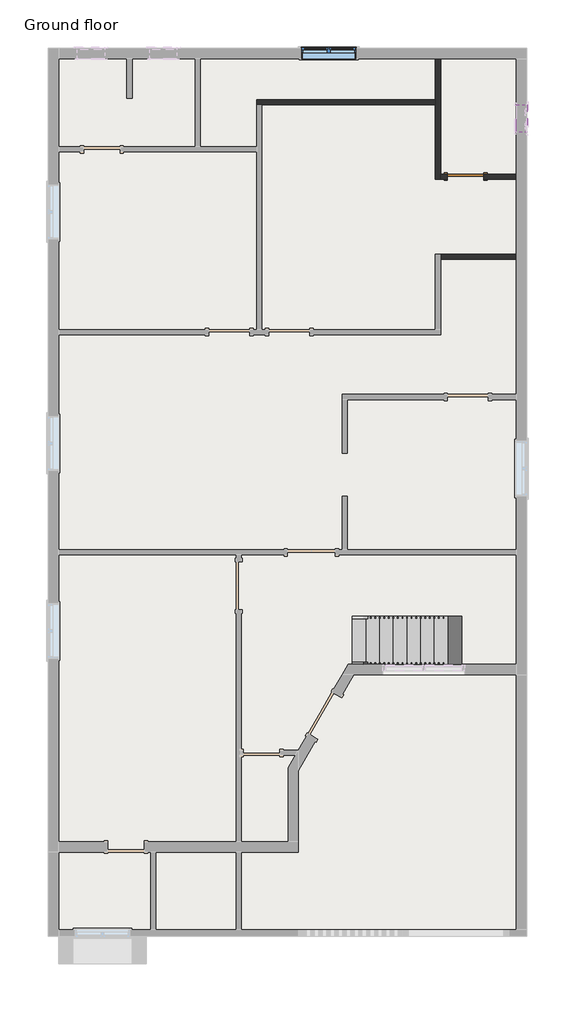
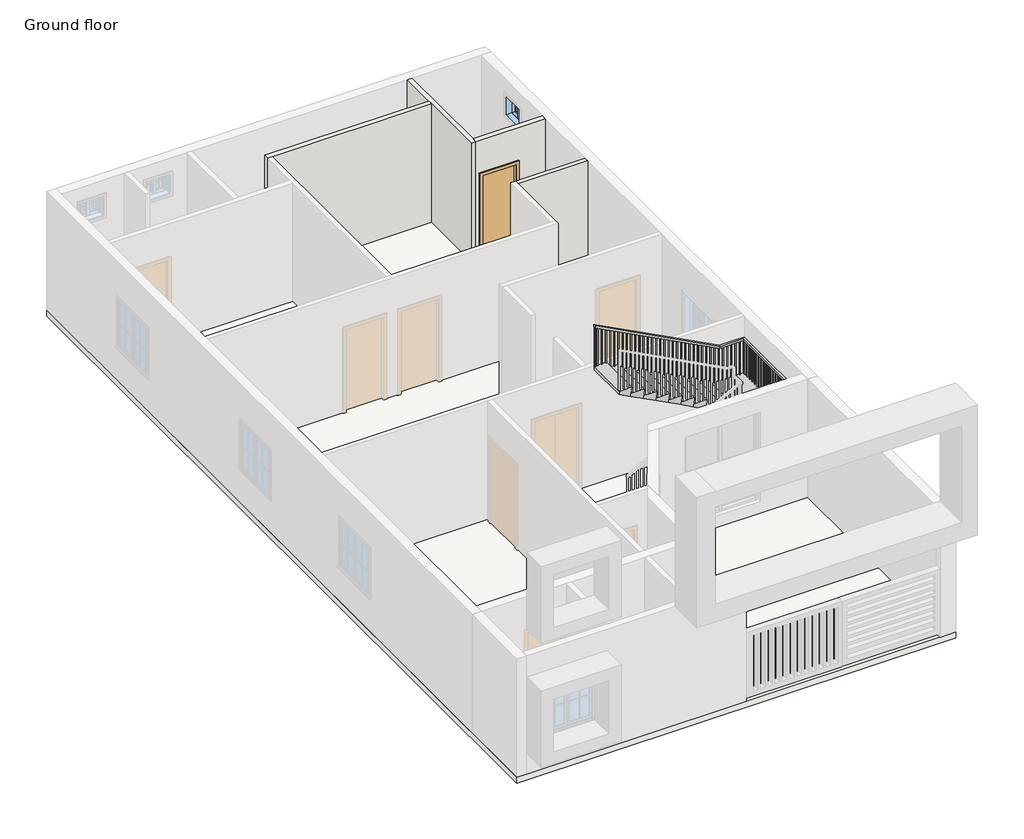
# One storey, part 2 of 3: 4 walls, 2 windows, 1 door, 1 railing, 1 slab, 1 stair flight.
"""IFC4 building model written with IfcOpenShell, lengths in millimetres."""

from ifc_helpers import new_model, si_unit, frame, origin, origin_with_axes, place, context, project, spatial, polyline, outline, extrude, faceted_brep, transform, mapped, element, save
from components import door_38851409, window_79894727, window_casement_double_4_x4_af3140d2

model = new_model("IFC4")

# Units and contexts
model_context = context("Model", 3, world=origin())
ifc_project = project(units=[si_unit("LENGTHUNIT", "METRE", prefix="MILLI")], contexts=[model_context])

# Site, building, storey
site = spatial("IfcSite", under=ifc_project)
building = spatial("IfcBuilding", under=site)
storey = spatial("IfcBuildingStorey", under=building, Name="Ground floor", Elevation=0.0)

# Door
placement = place(None, origin())
door_shape = door_38851409(model_context)
element("IfcDoor", 1, ObjectType="Single-Flush : 2'8\"X7'", at=placement, inside=storey, context=model_context, shape_type="MappedRepresentation", body=[
    mapped(door_shape, transform((3538.5585096, 7293.9976094, 0.0), x_axis=(-1.0, 0.0, 0.0), y_axis=(0.0, -1.0, 0.0), z_axis=(0.0, 0.0, 1.0))),
])

# Railing
element("IfcRailing", 2, ObjectType="Handrail - Rectangular", at=placement, inside=storey, context=model_context, shape_type="SolidModel", body=[
    faceted_brep([(1011.2585096, -3532.7523906, 1074.42), (1011.2585096, -3532.7523906, 1017.0446664), (1011.2585096, -3583.5523906, 1017.0446664), (1011.2585096, -3583.5523906, 1074.42), (3754.4585096, -3532.7523906, 2514.6), (3766.9829544, -3532.7523906, 2463.8), (3766.9829544, -3583.5523906, 2463.8), (3754.4585096, -3583.5523906, 2514.6), (4618.0585096, -3532.7523906, 2514.6), (4618.0585096, -3532.7523906, 2463.8), (4668.8585096, -3583.5523906, 2463.8), (4668.8585096, -3583.5523906, 2514.6), (4618.0585096, -1195.9523906, 2514.6), (4618.0585096, -1195.9523906, 2463.8), (4668.8585096, -1145.1523906, 2463.8), (4668.8585096, -1145.1523906, 2514.6), (4059.2585096, -1195.9523906, 2514.6), (4046.7340647, -1195.9523906, 2463.8), (4046.7340647, -1145.1523906, 2463.8), (4059.2585096, -1145.1523906, 2514.6), (1011.2585096, -1195.9523906, 4114.8), (1011.2585096, -1145.1523906, 4114.8), (1011.2585096, -1145.1523906, 4057.4246664), (1011.2585096, -1195.9523906, 4057.4246664)], [[[0, 1, 2, 3]], [[1, 0, 4, 5]], [[2, 1, 5, 6]], [[3, 2, 6, 7]], [[0, 3, 7, 4]], [[5, 4, 8, 9]], [[6, 5, 9, 10]], [[7, 6, 10, 11]], [[4, 7, 11, 8]], [[9, 8, 12, 13]], [[10, 9, 13, 14]], [[11, 10, 14, 15]], [[8, 11, 15, 12]], [[13, 12, 16, 17]], [[14, 13, 17, 18]], [[15, 14, 18, 19]], [[12, 15, 19, 16]], [[20, 21, 22, 23]], [[17, 16, 20, 23]], [[18, 17, 23, 22]], [[19, 18, 22, 21]], [[16, 19, 21, 20]]]),
    extrude(outline(polyline([(4012.4190414, 1096.9835096), (4022.4202914, 1077.9335096), (3040.38, 1077.9335096), (3040.38, 1096.9835096), (4012.4190414, 1096.9835096)])), frame((0.0, -1180.0773906, 0.0), z_axis=(0.0, 1.0, 0.0), x_axis=(0.0, 0.0, 1.0)), (0.0, 0.0, 1.0), 19.05),
    extrude(outline(polyline([(3959.0790414, 1198.5835096), (3969.0802914, 1179.5335096), (3040.38, 1179.5335096), (3040.38, 1198.5835096), (3959.0790414, 1198.5835096)])), frame((0.0, -1180.0773906, 0.0), z_axis=(0.0, 1.0, 0.0), x_axis=(0.0, 0.0, 1.0)), (0.0, 0.0, 1.0), 19.05),
    extrude(outline(polyline([(3905.7390414, 1300.1835096), (3915.7402914, 1281.1335096), (3040.38, 1281.1335096), (3040.38, 1300.1835096), (3905.7390414, 1300.1835096)])), frame((0.0, -1180.0773906, 0.0), z_axis=(0.0, 1.0, 0.0), x_axis=(0.0, 0.0, 1.0)), (0.0, 0.0, 1.0), 19.05),
    extrude(outline(polyline([(3852.3990414, 1401.7835096), (3862.4002914, 1382.7335096), (2880.36, 1382.7335096), (2880.36, 1401.7835096), (3852.3990414, 1401.7835096)])), frame((0.0, -1180.0773906, 0.0), z_axis=(0.0, 1.0, 0.0), x_axis=(0.0, 0.0, 1.0)), (0.0, 0.0, 1.0), 19.05),
    extrude(outline(polyline([(3799.0590414, 1503.3835096), (3809.0602914, 1484.3335096), (2880.36, 1484.3335096), (2880.36, 1503.3835096), (3799.0590414, 1503.3835096)])), frame((0.0, -1180.0773906, 0.0), z_axis=(0.0, 1.0, 0.0), x_axis=(0.0, 0.0, 1.0)), (0.0, 0.0, 1.0), 19.05),
    extrude(outline(polyline([(3745.7190414, 1604.9835096), (3755.7202914, 1585.9335096), (2880.36, 1585.9335096), (2880.36, 1604.9835096), (3745.7190414, 1604.9835096)])), frame((0.0, -1180.0773906, 0.0), z_axis=(0.0, 1.0, 0.0), x_axis=(0.0, 0.0, 1.0)), (0.0, 0.0, 1.0), 19.05),
    extrude(outline(polyline([(3692.3790414, 1706.5835096), (3702.3802914, 1687.5335096), (2720.34, 1687.5335096), (2720.34, 1706.5835096), (3692.3790414, 1706.5835096)])), frame((0.0, -1180.0773906, 0.0), z_axis=(0.0, 1.0, 0.0), x_axis=(0.0, 0.0, 1.0)), (0.0, 0.0, 1.0), 19.05),
    extrude(outline(polyline([(3639.0390414, 1808.1835096), (3649.0402914, 1789.1335096), (2720.34, 1789.1335096), (2720.34, 1808.1835096), (3639.0390414, 1808.1835096)])), frame((0.0, -1180.0773906, 0.0), z_axis=(0.0, 1.0, 0.0), x_axis=(0.0, 0.0, 1.0)), (0.0, 0.0, 1.0), 19.05),
    extrude(outline(polyline([(3585.6990414, 1909.7835096), (3595.7002914, 1890.7335096), (2720.34, 1890.7335096), (2720.34, 1909.7835096), (3585.6990414, 1909.7835096)])), frame((0.0, -1180.0773906, 0.0), z_axis=(0.0, 1.0, 0.0), x_axis=(0.0, 0.0, 1.0)), (0.0, 0.0, 1.0), 19.05),
    extrude(outline(polyline([(3532.3590414, 2011.3835096), (3542.3602914, 1992.3335096), (2560.32, 1992.3335096), (2560.32, 2011.3835096), (3532.3590414, 2011.3835096)])), frame((0.0, -1180.0773906, 0.0), z_axis=(0.0, 1.0, 0.0), x_axis=(0.0, 0.0, 1.0)), (0.0, 0.0, 1.0), 19.05),
    extrude(outline(polyline([(3479.0190414, 2112.9835096), (3489.0202914, 2093.9335096), (2560.32, 2093.9335096), (2560.32, 2112.9835096), (3479.0190414, 2112.9835096)])), frame((0.0, -1180.0773906, 0.0), z_axis=(0.0, 1.0, 0.0), x_axis=(0.0, 0.0, 1.0)), (0.0, 0.0, 1.0), 19.05),
    extrude(outline(polyline([(3425.6790414, 2214.5835096), (3435.6802914, 2195.5335096), (2560.32, 2195.5335096), (2560.32, 2214.5835096), (3425.6790414, 2214.5835096)])), frame((0.0, -1180.0773906, 0.0), z_axis=(0.0, 1.0, 0.0), x_axis=(0.0, 0.0, 1.0)), (0.0, 0.0, 1.0), 19.05),
    extrude(outline(polyline([(3372.3390414, 2316.1835096), (3382.3402914, 2297.1335096), (2400.3, 2297.1335096), (2400.3, 2316.1835096), (3372.3390414, 2316.1835096)])), frame((0.0, -1180.0773906, 0.0), z_axis=(0.0, 1.0, 0.0), x_axis=(0.0, 0.0, 1.0)), (0.0, 0.0, 1.0), 19.05),
    extrude(outline(polyline([(3318.9990414, 2417.7835096), (3329.0002914, 2398.7335096), (2400.3, 2398.7335096), (2400.3, 2417.7835096), (3318.9990414, 2417.7835096)])), frame((0.0, -1180.0773906, 0.0), z_axis=(0.0, 1.0, 0.0), x_axis=(0.0, 0.0, 1.0)), (0.0, 0.0, 1.0), 19.05),
    extrude(outline(polyline([(3265.6590414, 2519.3835096), (3275.6602914, 2500.3335096), (2400.3, 2500.3335096), (2400.3, 2519.3835096), (3265.6590414, 2519.3835096)])), frame((0.0, -1180.0773906, 0.0), z_axis=(0.0, 1.0, 0.0), x_axis=(0.0, 0.0, 1.0)), (0.0, 0.0, 1.0), 19.05),
    extrude(outline(polyline([(3212.3190414, 2620.9835096), (3222.3202914, 2601.9335096), (2240.28, 2601.9335096), (2240.28, 2620.9835096), (3212.3190414, 2620.9835096)])), frame((0.0, -1180.0773906, 0.0), z_axis=(0.0, 1.0, 0.0), x_axis=(0.0, 0.0, 1.0)), (0.0, 0.0, 1.0), 19.05),
    extrude(outline(polyline([(3158.9790414, 2722.5835096), (3168.9802914, 2703.5335096), (2240.28, 2703.5335096), (2240.28, 2722.5835096), (3158.9790414, 2722.5835096)])), frame((0.0, -1180.0773906, 0.0), z_axis=(0.0, 1.0, 0.0), x_axis=(0.0, 0.0, 1.0)), (0.0, 0.0, 1.0), 19.05),
    extrude(outline(polyline([(3105.6390414, 2824.1835096), (3115.6402914, 2805.1335096), (2240.28, 2805.1335096), (2240.28, 2824.1835096), (3105.6390414, 2824.1835096)])), frame((0.0, -1180.0773906, 0.0), z_axis=(0.0, 1.0, 0.0), x_axis=(0.0, 0.0, 1.0)), (0.0, 0.0, 1.0), 19.05),
    extrude(outline(polyline([(3052.2990414, 2925.7835096), (3062.3002914, 2906.7335096), (2080.26, 2906.7335096), (2080.26, 2925.7835096), (3052.2990414, 2925.7835096)])), frame((0.0, -1180.0773906, 0.0), z_axis=(0.0, 1.0, 0.0), x_axis=(0.0, 0.0, 1.0)), (0.0, 0.0, 1.0), 19.05),
    extrude(outline(polyline([(2998.9590414, 3027.3835096), (3008.9602914, 3008.3335096), (2080.26, 3008.3335096), (2080.26, 3027.3835096), (2998.9590414, 3027.3835096)])), frame((0.0, -1180.0773906, 0.0), z_axis=(0.0, 1.0, 0.0), x_axis=(0.0, 0.0, 1.0)), (0.0, 0.0, 1.0), 19.05),
    extrude(outline(polyline([(2945.6190414, 3128.9835096), (2955.6202914, 3109.9335096), (2080.26, 3109.9335096), (2080.26, 3128.9835096), (2945.6190414, 3128.9835096)])), frame((0.0, -1180.0773906, 0.0), z_axis=(0.0, 1.0, 0.0), x_axis=(0.0, 0.0, 1.0)), (0.0, 0.0, 1.0), 19.05),
    extrude(outline(polyline([(2892.2790414, 3230.5835096), (2902.2802914, 3211.5335096), (1920.24, 3211.5335096), (1920.24, 3230.5835096), (2892.2790414, 3230.5835096)])), frame((0.0, -1180.0773906, 0.0), z_axis=(0.0, 1.0, 0.0), x_axis=(0.0, 0.0, 1.0)), (0.0, 0.0, 1.0), 19.05),
    extrude(outline(polyline([(2838.9390414, 3332.1835096), (2848.9402914, 3313.1335096), (1920.24, 3313.1335096), (1920.24, 3332.1835096), (2838.9390414, 3332.1835096)])), frame((0.0, -1180.0773906, 0.0), z_axis=(0.0, 1.0, 0.0), x_axis=(0.0, 0.0, 1.0)), (0.0, 0.0, 1.0), 19.05),
    extrude(outline(polyline([(2785.5990414, 3433.7835096), (2795.6002914, 3414.7335096), (1920.24, 3414.7335096), (1920.24, 3433.7835096), (2785.5990414, 3433.7835096)])), frame((0.0, -1180.0773906, 0.0), z_axis=(0.0, 1.0, 0.0), x_axis=(0.0, 0.0, 1.0)), (0.0, 0.0, 1.0), 19.05),
    extrude(outline(polyline([(2732.2590414, 3535.3835096), (2742.2602914, 3516.3335096), (1760.22, 3516.3335096), (1760.22, 3535.3835096), (2732.2590414, 3535.3835096)])), frame((0.0, -1180.0773906, 0.0), z_axis=(0.0, 1.0, 0.0), x_axis=(0.0, 0.0, 1.0)), (0.0, 0.0, 1.0), 19.05),
    extrude(outline(polyline([(2678.9190414, 3636.9835096), (2688.9202914, 3617.9335096), (1760.22, 3617.9335096), (1760.22, 3636.9835096), (2678.9190414, 3636.9835096)])), frame((0.0, -1180.0773906, 0.0), z_axis=(0.0, 1.0, 0.0), x_axis=(0.0, 0.0, 1.0)), (0.0, 0.0, 1.0), 19.05),
    extrude(outline(polyline([(2625.5790414, 3738.5835096), (2635.5802914, 3719.5335096), (1760.22, 3719.5335096), (1760.22, 3738.5835096), (2625.5790414, 3738.5835096)])), frame((0.0, -1180.0773906, 0.0), z_axis=(0.0, 1.0, 0.0), x_axis=(0.0, 0.0, 1.0)), (0.0, 0.0, 1.0), 19.05),
    extrude(outline(polyline([(2572.2390414, 3840.1835096), (2582.2402914, 3821.1335096), (1600.2, 3821.1335096), (1600.2, 3840.1835096), (2572.2390414, 3840.1835096)])), frame((0.0, -1180.0773906, 0.0), z_axis=(0.0, 1.0, 0.0), x_axis=(0.0, 0.0, 1.0)), (0.0, 0.0, 1.0), 19.05),
    extrude(outline(polyline([(2518.8990414, 3941.7835096), (2528.9002914, 3922.7335096), (1600.2, 3922.7335096), (1600.2, 3941.7835096), (2518.8990414, 3941.7835096)])), frame((0.0, -1180.0773906, 0.0), z_axis=(0.0, 1.0, 0.0), x_axis=(0.0, 0.0, 1.0)), (0.0, 0.0, 1.0), 19.05),
    extrude(outline(polyline([(2465.5590414, 4043.3835096), (2475.5602914, 4024.3335096), (1600.2, 4024.3335096), (1600.2, 4043.3835096), (2465.5590414, 4043.3835096)])), frame((0.0, -1180.0773906, 0.0), z_axis=(0.0, 1.0, 0.0), x_axis=(0.0, 0.0, 1.0)), (0.0, 0.0, 1.0), 19.05),
    extrude(outline(polyline([(4144.9835096, -1161.0273906), (4144.9835096, -1180.0773906), (4125.9335096, -1180.0773906), (4125.9335096, -1161.0273906), (4144.9835096, -1161.0273906)])), frame((0.0, 0.0, 1600.2), z_axis=(0.0, 0.0, 1.0), x_axis=(1.0, 0.0, 0.0)), (0.0, 0.0, 1.0), 863.6),
    extrude(outline(polyline([(4246.5835096, -1161.0273906), (4246.5835096, -1180.0773906), (4227.5335096, -1180.0773906), (4227.5335096, -1161.0273906), (4246.5835096, -1161.0273906)])), frame((0.0, 0.0, 1600.2), z_axis=(0.0, 0.0, 1.0), x_axis=(1.0, 0.0, 0.0)), (0.0, 0.0, 1.0), 863.6),
    extrude(outline(polyline([(4348.1835096, -1161.0273906), (4348.1835096, -1180.0773906), (4329.1335096, -1180.0773906), (4329.1335096, -1161.0273906), (4348.1835096, -1161.0273906)])), frame((0.0, 0.0, 1600.2), z_axis=(0.0, 0.0, 1.0), x_axis=(1.0, 0.0, 0.0)), (0.0, 0.0, 1.0), 863.6),
    extrude(outline(polyline([(4449.7835096, -1161.0273906), (4449.7835096, -1180.0773906), (4430.7335096, -1180.0773906), (4430.7335096, -1161.0273906), (4449.7835096, -1161.0273906)])), frame((0.0, 0.0, 1600.2), z_axis=(0.0, 0.0, 1.0), x_axis=(1.0, 0.0, 0.0)), (0.0, 0.0, 1.0), 863.6),
    extrude(outline(polyline([(4551.3835096, -1161.0273906), (4551.3835096, -1180.0773906), (4532.3335096, -1180.0773906), (4532.3335096, -1161.0273906), (4551.3835096, -1161.0273906)])), frame((0.0, 0.0, 1600.2), z_axis=(0.0, 0.0, 1.0), x_axis=(1.0, 0.0, 0.0)), (0.0, 0.0, 1.0), 863.6),
    extrude(outline(polyline([(4652.9835096, -1230.8773906), (4633.9335096, -1230.8773906), (4633.9335096, -1211.8273906), (4652.9835096, -1211.8273906), (4652.9835096, -1230.8773906)])), frame((0.0, 0.0, 1600.2), z_axis=(0.0, 0.0, 1.0), x_axis=(1.0, 0.0, 0.0)), (0.0, 0.0, 1.0), 863.6),
    extrude(outline(polyline([(4652.9835096, -1332.4773906), (4633.9335096, -1332.4773906), (4633.9335096, -1313.4273906), (4652.9835096, -1313.4273906), (4652.9835096, -1332.4773906)])), frame((0.0, 0.0, 1600.2), z_axis=(0.0, 0.0, 1.0), x_axis=(1.0, 0.0, 0.0)), (0.0, 0.0, 1.0), 863.6),
    extrude(outline(polyline([(4652.9835096, -1434.0773906), (4633.9335096, -1434.0773906), (4633.9335096, -1415.0273906), (4652.9835096, -1415.0273906), (4652.9835096, -1434.0773906)])), frame((0.0, 0.0, 1600.2), z_axis=(0.0, 0.0, 1.0), x_axis=(1.0, 0.0, 0.0)), (0.0, 0.0, 1.0), 863.6),
    extrude(outline(polyline([(4652.9835096, -1535.6773906), (4633.9335096, -1535.6773906), (4633.9335096, -1516.6273906), (4652.9835096, -1516.6273906), (4652.9835096, -1535.6773906)])), frame((0.0, 0.0, 1600.2), z_axis=(0.0, 0.0, 1.0), x_axis=(1.0, 0.0, 0.0)), (0.0, 0.0, 1.0), 863.6),
    extrude(outline(polyline([(4652.9835096, -1637.2773906), (4633.9335096, -1637.2773906), (4633.9335096, -1618.2273906), (4652.9835096, -1618.2273906), (4652.9835096, -1637.2773906)])), frame((0.0, 0.0, 1600.2), z_axis=(0.0, 0.0, 1.0), x_axis=(1.0, 0.0, 0.0)), (0.0, 0.0, 1.0), 863.6),
    extrude(outline(polyline([(4652.9835096, -1738.8773906), (4633.9335096, -1738.8773906), (4633.9335096, -1719.8273906), (4652.9835096, -1719.8273906), (4652.9835096, -1738.8773906)])), frame((0.0, 0.0, 1600.2), z_axis=(0.0, 0.0, 1.0), x_axis=(1.0, 0.0, 0.0)), (0.0, 0.0, 1.0), 863.6),
    extrude(outline(polyline([(4652.9835096, -1840.4773906), (4633.9335096, -1840.4773906), (4633.9335096, -1821.4273906), (4652.9835096, -1821.4273906), (4652.9835096, -1840.4773906)])), frame((0.0, 0.0, 1600.2), z_axis=(0.0, 0.0, 1.0), x_axis=(1.0, 0.0, 0.0)), (0.0, 0.0, 1.0), 863.6),
    extrude(outline(polyline([(4652.9835096, -1942.0773906), (4633.9335096, -1942.0773906), (4633.9335096, -1923.0273906), (4652.9835096, -1923.0273906), (4652.9835096, -1942.0773906)])), frame((0.0, 0.0, 1600.2), z_axis=(0.0, 0.0, 1.0), x_axis=(1.0, 0.0, 0.0)), (0.0, 0.0, 1.0), 863.6),
    extrude(outline(polyline([(4652.9835096, -2043.6773906), (4633.9335096, -2043.6773906), (4633.9335096, -2024.6273906), (4652.9835096, -2024.6273906), (4652.9835096, -2043.6773906)])), frame((0.0, 0.0, 1600.2), z_axis=(0.0, 0.0, 1.0), x_axis=(1.0, 0.0, 0.0)), (0.0, 0.0, 1.0), 863.6),
    extrude(outline(polyline([(4652.9835096, -2145.2773906), (4633.9335096, -2145.2773906), (4633.9335096, -2126.2273906), (4652.9835096, -2126.2273906), (4652.9835096, -2145.2773906)])), frame((0.0, 0.0, 1600.2), z_axis=(0.0, 0.0, 1.0), x_axis=(1.0, 0.0, 0.0)), (0.0, 0.0, 1.0), 863.6),
    extrude(outline(polyline([(4652.9835096, -2246.8773906), (4633.9335096, -2246.8773906), (4633.9335096, -2227.8273906), (4652.9835096, -2227.8273906), (4652.9835096, -2246.8773906)])), frame((0.0, 0.0, 1600.2), z_axis=(0.0, 0.0, 1.0), x_axis=(1.0, 0.0, 0.0)), (0.0, 0.0, 1.0), 863.6),
    extrude(outline(polyline([(4652.9835096, -2348.4773906), (4633.9335096, -2348.4773906), (4633.9335096, -2329.4273906), (4652.9835096, -2329.4273906), (4652.9835096, -2348.4773906)])), frame((0.0, 0.0, 1600.2), z_axis=(0.0, 0.0, 1.0), x_axis=(1.0, 0.0, 0.0)), (0.0, 0.0, 1.0), 863.6),
    extrude(outline(polyline([(4652.9835096, -2450.0773906), (4633.9335096, -2450.0773906), (4633.9335096, -2431.0273906), (4652.9835096, -2431.0273906), (4652.9835096, -2450.0773906)])), frame((0.0, 0.0, 1600.2), z_axis=(0.0, 0.0, 1.0), x_axis=(1.0, 0.0, 0.0)), (0.0, 0.0, 1.0), 863.6),
    extrude(outline(polyline([(4652.9835096, -2551.6773906), (4633.9335096, -2551.6773906), (4633.9335096, -2532.6273906), (4652.9835096, -2532.6273906), (4652.9835096, -2551.6773906)])), frame((0.0, 0.0, 1600.2), z_axis=(0.0, 0.0, 1.0), x_axis=(1.0, 0.0, 0.0)), (0.0, 0.0, 1.0), 863.6),
    extrude(outline(polyline([(4652.9835096, -2653.2773906), (4633.9335096, -2653.2773906), (4633.9335096, -2634.2273906), (4652.9835096, -2634.2273906), (4652.9835096, -2653.2773906)])), frame((0.0, 0.0, 1600.2), z_axis=(0.0, 0.0, 1.0), x_axis=(1.0, 0.0, 0.0)), (0.0, 0.0, 1.0), 863.6),
    extrude(outline(polyline([(4652.9835096, -2754.8773906), (4633.9335096, -2754.8773906), (4633.9335096, -2735.8273906), (4652.9835096, -2735.8273906), (4652.9835096, -2754.8773906)])), frame((0.0, 0.0, 1600.2), z_axis=(0.0, 0.0, 1.0), x_axis=(1.0, 0.0, 0.0)), (0.0, 0.0, 1.0), 863.6),
    extrude(outline(polyline([(4652.9835096, -2856.4773906), (4633.9335096, -2856.4773906), (4633.9335096, -2837.4273906), (4652.9835096, -2837.4273906), (4652.9835096, -2856.4773906)])), frame((0.0, 0.0, 1600.2), z_axis=(0.0, 0.0, 1.0), x_axis=(1.0, 0.0, 0.0)), (0.0, 0.0, 1.0), 863.6),
    extrude(outline(polyline([(4652.9835096, -2958.0773906), (4633.9335096, -2958.0773906), (4633.9335096, -2939.0273906), (4652.9835096, -2939.0273906), (4652.9835096, -2958.0773906)])), frame((0.0, 0.0, 1600.2), z_axis=(0.0, 0.0, 1.0), x_axis=(1.0, 0.0, 0.0)), (0.0, 0.0, 1.0), 863.6),
    extrude(outline(polyline([(4652.9835096, -3059.6773906), (4633.9335096, -3059.6773906), (4633.9335096, -3040.6273906), (4652.9835096, -3040.6273906), (4652.9835096, -3059.6773906)])), frame((0.0, 0.0, 1600.2), z_axis=(0.0, 0.0, 1.0), x_axis=(1.0, 0.0, 0.0)), (0.0, 0.0, 1.0), 863.6),
    extrude(outline(polyline([(4652.9835096, -3161.2773906), (4633.9335096, -3161.2773906), (4633.9335096, -3142.2273906), (4652.9835096, -3142.2273906), (4652.9835096, -3161.2773906)])), frame((0.0, 0.0, 1600.2), z_axis=(0.0, 0.0, 1.0), x_axis=(1.0, 0.0, 0.0)), (0.0, 0.0, 1.0), 863.6),
    extrude(outline(polyline([(4652.9835096, -3262.8773906), (4633.9335096, -3262.8773906), (4633.9335096, -3243.8273906), (4652.9835096, -3243.8273906), (4652.9835096, -3262.8773906)])), frame((0.0, 0.0, 1600.2), z_axis=(0.0, 0.0, 1.0), x_axis=(1.0, 0.0, 0.0)), (0.0, 0.0, 1.0), 863.6),
    extrude(outline(polyline([(4652.9835096, -3364.4773906), (4633.9335096, -3364.4773906), (4633.9335096, -3345.4273906), (4652.9835096, -3345.4273906), (4652.9835096, -3364.4773906)])), frame((0.0, 0.0, 1600.2), z_axis=(0.0, 0.0, 1.0), x_axis=(1.0, 0.0, 0.0)), (0.0, 0.0, 1.0), 863.6),
    extrude(outline(polyline([(4652.9835096, -3466.0773906), (4633.9335096, -3466.0773906), (4633.9335096, -3447.0273906), (4652.9835096, -3447.0273906), (4652.9835096, -3466.0773906)])), frame((0.0, 0.0, 1600.2), z_axis=(0.0, 0.0, 1.0), x_axis=(1.0, 0.0, 0.0)), (0.0, 0.0, 1.0), 863.6),
    extrude(outline(polyline([(4557.7335096, -3567.6773906), (4557.7335096, -3548.6273906), (4576.7835096, -3548.6273906), (4576.7835096, -3567.6773906), (4557.7335096, -3567.6773906)])), frame((0.0, 0.0, 1600.2), z_axis=(0.0, 0.0, 1.0), x_axis=(1.0, 0.0, 0.0)), (0.0, 0.0, 1.0), 863.6),
    extrude(outline(polyline([(4456.1335096, -3567.6773906), (4456.1335096, -3548.6273906), (4475.1835096, -3548.6273906), (4475.1835096, -3567.6773906), (4456.1335096, -3567.6773906)])), frame((0.0, 0.0, 1600.2), z_axis=(0.0, 0.0, 1.0), x_axis=(1.0, 0.0, 0.0)), (0.0, 0.0, 1.0), 863.6),
    extrude(outline(polyline([(4354.5335096, -3567.6773906), (4354.5335096, -3548.6273906), (4373.5835096, -3548.6273906), (4373.5835096, -3567.6773906), (4354.5335096, -3567.6773906)])), frame((0.0, 0.0, 1600.2), z_axis=(0.0, 0.0, 1.0), x_axis=(1.0, 0.0, 0.0)), (0.0, 0.0, 1.0), 863.6),
    extrude(outline(polyline([(4252.9335096, -3567.6773906), (4252.9335096, -3548.6273906), (4271.9835096, -3548.6273906), (4271.9835096, -3567.6773906), (4252.9335096, -3567.6773906)])), frame((0.0, 0.0, 1600.2), z_axis=(0.0, 0.0, 1.0), x_axis=(1.0, 0.0, 0.0)), (0.0, 0.0, 1.0), 863.6),
    extrude(outline(polyline([(4151.3335096, -3567.6773906), (4151.3335096, -3548.6273906), (4170.3835096, -3548.6273906), (4170.3835096, -3567.6773906), (4151.3335096, -3567.6773906)])), frame((0.0, 0.0, 1600.2), z_axis=(0.0, 0.0, 1.0), x_axis=(1.0, 0.0, 0.0)), (0.0, 0.0, 1.0), 863.6),
    extrude(outline(polyline([(4049.7335096, -3567.6773906), (4049.7335096, -3548.6273906), (4068.7835096, -3548.6273906), (4068.7835096, -3567.6773906), (4049.7335096, -3567.6773906)])), frame((0.0, 0.0, 1600.2), z_axis=(0.0, 0.0, 1.0), x_axis=(1.0, 0.0, 0.0)), (0.0, 0.0, 1.0), 863.6),
    extrude(outline(polyline([(3948.1335096, -3567.6773906), (3948.1335096, -3548.6273906), (3967.1835096, -3548.6273906), (3967.1835096, -3567.6773906), (3948.1335096, -3567.6773906)])), frame((0.0, 0.0, 1600.2), z_axis=(0.0, 0.0, 1.0), x_axis=(1.0, 0.0, 0.0)), (0.0, 0.0, 1.0), 863.6),
    extrude(outline(polyline([(3846.5335096, -3567.6773906), (3846.5335096, -3548.6273906), (3865.5835096, -3548.6273906), (3865.5835096, -3567.6773906), (3846.5335096, -3567.6773906)])), frame((0.0, 0.0, 1600.2), z_axis=(0.0, 0.0, 1.0), x_axis=(1.0, 0.0, 0.0)), (0.0, 0.0, 1.0), 863.6),
    extrude(outline(polyline([(2462.2252914, 3763.9835096), (2452.2240414, 3744.9335096), (1600.2, 3744.9335096), (1600.2, 3763.9835096), (2462.2252914, 3763.9835096)])), frame((0.0, -3567.6773906, 0.0), z_axis=(0.0, 1.0, 0.0), x_axis=(0.0, 0.0, 1.0)), (0.0, 0.0, 1.0), 19.05),
    extrude(outline(polyline([(2408.8852914, 3662.3835096), (2398.8840414, 3643.3335096), (1440.18, 3643.3335096), (1440.18, 3662.3835096), (2408.8852914, 3662.3835096)])), frame((0.0, -3567.6773906, 0.0), z_axis=(0.0, 1.0, 0.0), x_axis=(0.0, 0.0, 1.0)), (0.0, 0.0, 1.0), 19.05),
    extrude(outline(polyline([(2355.5452914, 3560.7835096), (2345.5440414, 3541.7335096), (1440.18, 3541.7335096), (1440.18, 3560.7835096), (2355.5452914, 3560.7835096)])), frame((0.0, -3567.6773906, 0.0), z_axis=(0.0, 1.0, 0.0), x_axis=(0.0, 0.0, 1.0)), (0.0, 0.0, 1.0), 19.05),
    extrude(outline(polyline([(2302.2052914, 3459.1835096), (2292.2040414, 3440.1335096), (1440.18, 3440.1335096), (1440.18, 3459.1835096), (2302.2052914, 3459.1835096)])), frame((0.0, -3567.6773906, 0.0), z_axis=(0.0, 1.0, 0.0), x_axis=(0.0, 0.0, 1.0)), (0.0, 0.0, 1.0), 19.05),
    extrude(outline(polyline([(2248.8652914, 3357.5835096), (2238.8640414, 3338.5335096), (1280.16, 3338.5335096), (1280.16, 3357.5835096), (2248.8652914, 3357.5835096)])), frame((0.0, -3567.6773906, 0.0), z_axis=(0.0, 1.0, 0.0), x_axis=(0.0, 0.0, 1.0)), (0.0, 0.0, 1.0), 19.05),
    extrude(outline(polyline([(2195.5252914, 3255.9835096), (2185.5240414, 3236.9335096), (1280.16, 3236.9335096), (1280.16, 3255.9835096), (2195.5252914, 3255.9835096)])), frame((0.0, -3567.6773906, 0.0), z_axis=(0.0, 1.0, 0.0), x_axis=(0.0, 0.0, 1.0)), (0.0, 0.0, 1.0), 19.05),
    extrude(outline(polyline([(2142.1852914, 3154.3835096), (2132.1840414, 3135.3335096), (1280.16, 3135.3335096), (1280.16, 3154.3835096), (2142.1852914, 3154.3835096)])), frame((0.0, -3567.6773906, 0.0), z_axis=(0.0, 1.0, 0.0), x_axis=(0.0, 0.0, 1.0)), (0.0, 0.0, 1.0), 19.05),
    extrude(outline(polyline([(2088.8452914, 3052.7835096), (2078.8440414, 3033.7335096), (1120.14, 3033.7335096), (1120.14, 3052.7835096), (2088.8452914, 3052.7835096)])), frame((0.0, -3567.6773906, 0.0), z_axis=(0.0, 1.0, 0.0), x_axis=(0.0, 0.0, 1.0)), (0.0, 0.0, 1.0), 19.05),
    extrude(outline(polyline([(2035.5052914, 2951.1835096), (2025.5040414, 2932.1335096), (1120.14, 2932.1335096), (1120.14, 2951.1835096), (2035.5052914, 2951.1835096)])), frame((0.0, -3567.6773906, 0.0), z_axis=(0.0, 1.0, 0.0), x_axis=(0.0, 0.0, 1.0)), (0.0, 0.0, 1.0), 19.05),
    extrude(outline(polyline([(1982.1652914, 2849.5835096), (1972.1640414, 2830.5335096), (1120.14, 2830.5335096), (1120.14, 2849.5835096), (1982.1652914, 2849.5835096)])), frame((0.0, -3567.6773906, 0.0), z_axis=(0.0, 1.0, 0.0), x_axis=(0.0, 0.0, 1.0)), (0.0, 0.0, 1.0), 19.05),
    extrude(outline(polyline([(1928.8252914, 2747.9835096), (1918.8240414, 2728.9335096), (960.12, 2728.9335096), (960.12, 2747.9835096), (1928.8252914, 2747.9835096)])), frame((0.0, -3567.6773906, 0.0), z_axis=(0.0, 1.0, 0.0), x_axis=(0.0, 0.0, 1.0)), (0.0, 0.0, 1.0), 19.05),
    extrude(outline(polyline([(1875.4852914, 2646.3835096), (1865.4840414, 2627.3335096), (960.12, 2627.3335096), (960.12, 2646.3835096), (1875.4852914, 2646.3835096)])), frame((0.0, -3567.6773906, 0.0), z_axis=(0.0, 1.0, 0.0), x_axis=(0.0, 0.0, 1.0)), (0.0, 0.0, 1.0), 19.05),
    extrude(outline(polyline([(1822.1452914, 2544.7835096), (1812.1440414, 2525.7335096), (960.12, 2525.7335096), (960.12, 2544.7835096), (1822.1452914, 2544.7835096)])), frame((0.0, -3567.6773906, 0.0), z_axis=(0.0, 1.0, 0.0), x_axis=(0.0, 0.0, 1.0)), (0.0, 0.0, 1.0), 19.05),
    extrude(outline(polyline([(1768.8052914, 2443.1835096), (1758.8040414, 2424.1335096), (800.1, 2424.1335096), (800.1, 2443.1835096), (1768.8052914, 2443.1835096)])), frame((0.0, -3567.6773906, 0.0), z_axis=(0.0, 1.0, 0.0), x_axis=(0.0, 0.0, 1.0)), (0.0, 0.0, 1.0), 19.05),
    extrude(outline(polyline([(1715.4652914, 2341.5835096), (1705.4640414, 2322.5335096), (800.1, 2322.5335096), (800.1, 2341.5835096), (1715.4652914, 2341.5835096)])), frame((0.0, -3567.6773906, 0.0), z_axis=(0.0, 1.0, 0.0), x_axis=(0.0, 0.0, 1.0)), (0.0, 0.0, 1.0), 19.05),
    extrude(outline(polyline([(1662.1252914, 2239.9835096), (1652.1240414, 2220.9335096), (800.1, 2220.9335096), (800.1, 2239.9835096), (1662.1252914, 2239.9835096)])), frame((0.0, -3567.6773906, 0.0), z_axis=(0.0, 1.0, 0.0), x_axis=(0.0, 0.0, 1.0)), (0.0, 0.0, 1.0), 19.05),
    extrude(outline(polyline([(1608.7852914, 2138.3835096), (1598.7840414, 2119.3335096), (640.08, 2119.3335096), (640.08, 2138.3835096), (1608.7852914, 2138.3835096)])), frame((0.0, -3567.6773906, 0.0), z_axis=(0.0, 1.0, 0.0), x_axis=(0.0, 0.0, 1.0)), (0.0, 0.0, 1.0), 19.05),
    extrude(outline(polyline([(1555.4452914, 2036.7835096), (1545.4440414, 2017.7335096), (640.08, 2017.7335096), (640.08, 2036.7835096), (1555.4452914, 2036.7835096)])), frame((0.0, -3567.6773906, 0.0), z_axis=(0.0, 1.0, 0.0), x_axis=(0.0, 0.0, 1.0)), (0.0, 0.0, 1.0), 19.05),
    extrude(outline(polyline([(1502.1052914, 1935.1835096), (1492.1040414, 1916.1335096), (640.08, 1916.1335096), (640.08, 1935.1835096), (1502.1052914, 1935.1835096)])), frame((0.0, -3567.6773906, 0.0), z_axis=(0.0, 1.0, 0.0), x_axis=(0.0, 0.0, 1.0)), (0.0, 0.0, 1.0), 19.05),
    extrude(outline(polyline([(1448.7652914, 1833.5835096), (1438.7640414, 1814.5335096), (480.06, 1814.5335096), (480.06, 1833.5835096), (1448.7652914, 1833.5835096)])), frame((0.0, -3567.6773906, 0.0), z_axis=(0.0, 1.0, 0.0), x_axis=(0.0, 0.0, 1.0)), (0.0, 0.0, 1.0), 19.05),
    extrude(outline(polyline([(1395.4252914, 1731.9835096), (1385.4240414, 1712.9335096), (480.06, 1712.9335096), (480.06, 1731.9835096), (1395.4252914, 1731.9835096)])), frame((0.0, -3567.6773906, 0.0), z_axis=(0.0, 1.0, 0.0), x_axis=(0.0, 0.0, 1.0)), (0.0, 0.0, 1.0), 19.05),
    extrude(outline(polyline([(1342.0852914, 1630.3835096), (1332.0840414, 1611.3335096), (480.06, 1611.3335096), (480.06, 1630.3835096), (1342.0852914, 1630.3835096)])), frame((0.0, -3567.6773906, 0.0), z_axis=(0.0, 1.0, 0.0), x_axis=(0.0, 0.0, 1.0)), (0.0, 0.0, 1.0), 19.05),
    extrude(outline(polyline([(1288.7452914, 1528.7835096), (1278.7440414, 1509.7335096), (320.04, 1509.7335096), (320.04, 1528.7835096), (1288.7452914, 1528.7835096)])), frame((0.0, -3567.6773906, 0.0), z_axis=(0.0, 1.0, 0.0), x_axis=(0.0, 0.0, 1.0)), (0.0, 0.0, 1.0), 19.05),
    extrude(outline(polyline([(1235.4052914, 1427.1835096), (1225.4040414, 1408.1335096), (320.04, 1408.1335096), (320.04, 1427.1835096), (1235.4052914, 1427.1835096)])), frame((0.0, -3567.6773906, 0.0), z_axis=(0.0, 1.0, 0.0), x_axis=(0.0, 0.0, 1.0)), (0.0, 0.0, 1.0), 19.05),
    extrude(outline(polyline([(1182.0652914, 1325.5835096), (1172.0640414, 1306.5335096), (320.04, 1306.5335096), (320.04, 1325.5835096), (1182.0652914, 1325.5835096)])), frame((0.0, -3567.6773906, 0.0), z_axis=(0.0, 1.0, 0.0), x_axis=(0.0, 0.0, 1.0)), (0.0, 0.0, 1.0), 19.05),
    extrude(outline(polyline([(1128.7252914, 1223.9835096), (1118.7240414, 1204.9335096), (160.02, 1204.9335096), (160.02, 1223.9835096), (1128.7252914, 1223.9835096)])), frame((0.0, -3567.6773906, 0.0), z_axis=(0.0, 1.0, 0.0), x_axis=(0.0, 0.0, 1.0)), (0.0, 0.0, 1.0), 19.05),
    extrude(outline(polyline([(1075.3852914, 1122.3835096), (1065.3840414, 1103.3335096), (160.02, 1103.3335096), (160.02, 1122.3835096), (1075.3852914, 1122.3835096)])), frame((0.0, -3567.6773906, 0.0), z_axis=(0.0, 1.0, 0.0), x_axis=(0.0, 0.0, 1.0)), (0.0, 0.0, 1.0), 19.05),
    extrude(outline(polyline([(4652.9835096, -1180.0773906), (4633.9335096, -1180.0773906), (4633.9335096, -1161.0273906), (4652.9835096, -1161.0273906), (4652.9835096, -1180.0773906)])), frame((0.0, 0.0, 1600.2), z_axis=(0.0, 0.0, 1.0), x_axis=(1.0, 0.0, 0.0)), (0.0, 0.0, 1.0), 863.6),
    extrude(outline(polyline([(4633.9335096, -3567.6773906), (4633.9335096, -3548.6273906), (4652.9835096, -3548.6273906), (4652.9835096, -3567.6773906), (4633.9335096, -3567.6773906)])), frame((0.0, 0.0, 1600.2), z_axis=(0.0, 0.0, 1.0), x_axis=(1.0, 0.0, 0.0)), (0.0, 0.0, 1.0), 863.6),
    extrude(outline(polyline([(4047.4234164, 1030.3085096), (4057.4246664, 1011.2585096), (3040.38, 1011.2585096), (3040.38, 1030.3085096), (4047.4234164, 1030.3085096)])), frame((0.0, -1180.0773906, 0.0), z_axis=(0.0, 1.0, 0.0), x_axis=(0.0, 0.0, 1.0)), (0.0, 0.0, 1.0), 19.05),
    extrude(outline(polyline([(1027.0459164, 1030.3085096), (1017.0446664, 1011.2585096), (160.02, 1011.2585096), (160.02, 1030.3085096), (1027.0459164, 1030.3085096)])), frame((0.0, -3567.6773906, 0.0), z_axis=(0.0, 1.0, 0.0), x_axis=(0.0, 0.0, 1.0)), (0.0, 0.0, 1.0), 19.05),
])

# Slab
element("IfcSlab", 3, ObjectType="6\"", at=placement, inside=storey, context=model_context, shape_type="SweptSolid", body=[
    extrude(outline(polyline([(4897.4585096, 10157.8476094), (4897.4585096, -9654.1523906), (-5772.1289904, -9654.1523906), (-5772.1289904, 10157.8476094), (4897.4585096, 10157.8476094)])), frame((0.0, 0.0, -152.4), z_axis=(0.0, 0.0, 1.0), x_axis=(1.0, 0.0, 0.0)), (0.0, 0.0, 1.0), 152.4),
])

# Stair flight
element("IfcStairFlight", 4, ObjectType="3/4\" Nosing", at=placement, inside=storey, context=model_context, shape_type="Brep", body=[
    faceted_brep([(1011.2585096, -2516.7523906, 160.02), (1011.2585096, -3583.5523906, 160.02), (1335.1085096, -3583.5523906, 160.02), (1335.1085096, -2516.7523906, 160.02), (1335.1085096, -2516.7523906, 88.3008331), (1166.9164466, -2516.7523906, 0.0), (1030.3085096, -2516.7523906, 0.0), (1030.3085096, -3583.5523906, 0.0), (1166.9164466, -3583.5523906, 0.0), (1335.1085096, -3583.5523906, 88.3008331), (1316.0585096, -2516.7523906, 320.04), (1316.0585096, -3583.5523906, 320.04), (1639.9085096, -3583.5523906, 320.04), (1639.9085096, -2516.7523906, 320.04), (1639.9085096, -2516.7523906, 248.3208331), (1639.9085096, -3583.5523906, 248.3208331), (1620.8585096, -2516.7523906, 480.06), (1620.8585096, -3583.5523906, 480.06), (1944.7085096, -3583.5523906, 480.06), (1944.7085096, -2516.7523906, 480.06), (1944.7085096, -2516.7523906, 408.3408331), (1944.7085096, -3583.5523906, 408.3408331), (1925.6585096, -2516.7523906, 640.08), (1925.6585096, -3583.5523906, 640.08), (2249.5085096, -3583.5523906, 640.08), (2249.5085096, -2516.7523906, 640.08), (2249.5085096, -2516.7523906, 568.3608331), (2249.5085096, -3583.5523906, 568.3608331), (2230.4585096, -2516.7523906, 800.1), (2230.4585096, -3583.5523906, 800.1), (2554.3085096, -3583.5523906, 800.1), (2554.3085096, -2516.7523906, 800.1), (2554.3085096, -2516.7523906, 728.3808331), (2554.3085096, -3583.5523906, 728.3808331), (2535.2585096, -2516.7523906, 960.12), (2535.2585096, -3583.5523906, 960.12), (2859.1085096, -3583.5523906, 960.12), (2859.1085096, -2516.7523906, 960.12), (2859.1085096, -2516.7523906, 888.4008331), (2859.1085096, -3583.5523906, 888.4008331), (2840.0585096, -2516.7523906, 1120.14), (2840.0585096, -3583.5523906, 1120.14), (3163.9085096, -3583.5523906, 1120.14), (3163.9085096, -2516.7523906, 1120.14), (3163.9085096, -2516.7523906, 1048.4208331), (3163.9085096, -3583.5523906, 1048.4208331), (3144.8585096, -2516.7523906, 1280.16), (3144.8585096, -3583.5523906, 1280.16), (3468.7085096, -3583.5523906, 1280.16), (3468.7085096, -2516.7523906, 1280.16), (3468.7085096, -2516.7523906, 1208.4408331), (3468.7085096, -3583.5523906, 1208.4408331), (3773.5085096, -2516.7523906, 1440.18), (3449.6585096, -2516.7523906, 1440.18), (3449.6585096, -3583.5523906, 1440.18), (3773.5085096, -3583.5523906, 1440.18), (3762.0180334, -2516.7523906, 1536.7), (4093.9640656, -2516.7523906, 1536.7), (3773.5085096, -3583.5523906, 1368.4608331), (3735.4085096, -2211.9523906, 1600.2), (3754.4585096, -2211.9523906, 1600.2), (3754.4585096, -2516.7523906, 1600.2), (3754.4585096, -3583.5523906, 1600.2), (4093.9640656, -3583.5523906, 1600.2), (4668.8585096, -3583.5523906, 1600.2), (4668.8585096, -1145.1523906, 1600.2), (3735.4085096, -1145.1523906, 1600.2), (3735.4085096, -2211.9523906, 1536.7), (3754.4585096, -2211.9523906, 1536.7), (3754.4585096, -2516.7523906, 1536.7), (4093.9640656, -3583.5523906, 1536.7), (4668.8585096, -3583.5523906, 1536.7), (4668.8585096, -1145.1523906, 1536.7), (3735.4085096, -1145.1523906, 1536.7), (3754.4585096, -2211.9523906, 1760.22), (3754.4585096, -1145.1523906, 1760.22), (3719.7529535, -1145.1523906, 1760.22), (3430.6085096, -1145.1523906, 1760.22), (3430.6085096, -2211.9523906, 1760.22), (3719.7529535, -2211.9523906, 1760.22), (3430.6085096, -2211.9523906, 1688.5008331), (3719.7529535, -2211.9523906, 1536.7), (3719.7529535, -1145.1523906, 1536.7), (3430.6085096, -1145.1523906, 1688.5008331), (3449.6585096, -2211.9523906, 1920.24), (3449.6585096, -1145.1523906, 1920.24), (3125.8085096, -1145.1523906, 1920.24), (3125.8085096, -2211.9523906, 1920.24), (3125.8085096, -2211.9523906, 1848.5208331), (3125.8085096, -1145.1523906, 1848.5208331), (3144.8585096, -2211.9523906, 2080.26), (3144.8585096, -1145.1523906, 2080.26), (2821.0085096, -1145.1523906, 2080.26), (2821.0085096, -2211.9523906, 2080.26), (2821.0085096, -2211.9523906, 2008.5408331), (2821.0085096, -1145.1523906, 2008.5408331), (2840.0585096, -2211.9523906, 2240.28), (2840.0585096, -1145.1523906, 2240.28), (2516.2085096, -1145.1523906, 2240.28), (2516.2085096, -2211.9523906, 2240.28), (2516.2085096, -2211.9523906, 2168.5608331), (2516.2085096, -1145.1523906, 2168.5608331), (2535.2585096, -2211.9523906, 2400.3), (2535.2585096, -1145.1523906, 2400.3), (2211.4085096, -1145.1523906, 2400.3), (2211.4085096, -2211.9523906, 2400.3), (2211.4085096, -2211.9523906, 2328.5808331), (2211.4085096, -1145.1523906, 2328.5808331), (2230.4585096, -2211.9523906, 2560.32), (2230.4585096, -1145.1523906, 2560.32), (1906.6085096, -1145.1523906, 2560.32), (1906.6085096, -2211.9523906, 2560.32), (1906.6085096, -2211.9523906, 2488.6008331), (1906.6085096, -1145.1523906, 2488.6008331), (1925.6585096, -2211.9523906, 2720.34), (1925.6585096, -1145.1523906, 2720.34), (1601.8085096, -1145.1523906, 2720.34), (1601.8085096, -2211.9523906, 2720.34), (1601.8085096, -2211.9523906, 2648.6208331), (1601.8085096, -1145.1523906, 2648.6208331), (1620.8585096, -2211.9523906, 2880.36), (1620.8585096, -1145.1523906, 2880.36), (1297.0085096, -1145.1523906, 2880.36), (1297.0085096, -2211.9523906, 2880.36), (1297.0085096, -2211.9523906, 2808.6408331), (1297.0085096, -1145.1523906, 2808.6408331), (1316.0585096, -2211.9523906, 3040.38), (1316.0585096, -1145.1523906, 3040.38), (1011.2585096, -1145.1523906, 3040.38), (1011.2585096, -2211.9523906, 3040.38), (1011.2585096, -2211.9523906, 2958.6595831), (1011.2585096, -1145.1523906, 2958.6595831)], [[[0, 1, 2, 3]], [[0, 3, 4, 5, 6]], [[2, 1, 7, 8, 9]], [[10, 11, 12, 13]], [[10, 13, 14, 4, 3]], [[12, 11, 2, 9, 15]], [[16, 17, 18, 19]], [[16, 19, 20, 14, 13]], [[18, 17, 12, 15, 21]], [[22, 23, 24, 25]], [[22, 25, 26, 20, 19]], [[24, 23, 18, 21, 27]], [[28, 29, 30, 31]], [[28, 31, 32, 26, 25]], [[30, 29, 24, 27, 33]], [[34, 35, 36, 37]], [[34, 37, 38, 32, 31]], [[36, 35, 30, 33, 39]], [[40, 41, 42, 43]], [[40, 43, 44, 38, 37]], [[42, 41, 36, 39, 45]], [[46, 47, 48, 49]], [[46, 49, 50, 44, 43]], [[48, 47, 42, 45, 51]], [[52, 53, 54, 55]], [[52, 56, 57, 50, 49, 53]], [[55, 54, 48, 51, 58]], [[59, 60, 61, 62, 63, 64, 65, 66]], [[60, 59, 67, 68]], [[61, 60, 68, 69]], [[56, 61, 69]], [[62, 55, 58, 70, 71, 64, 63]], [[65, 64, 71, 72]], [[66, 65, 72, 73]], [[74, 75, 76, 77, 78, 79]], [[59, 74, 79, 78, 80, 81, 67]], [[75, 66, 73, 82, 83, 77, 76]], [[84, 85, 86, 87]], [[84, 87, 88, 80, 78]], [[86, 85, 77, 83, 89]], [[90, 91, 92, 93]], [[90, 93, 94, 88, 87]], [[92, 91, 86, 89, 95]], [[96, 97, 98, 99]], [[96, 99, 100, 94, 93]], [[98, 97, 92, 95, 101]], [[102, 103, 104, 105]], [[102, 105, 106, 100, 99]], [[104, 103, 98, 101, 107]], [[108, 109, 110, 111]], [[108, 111, 112, 106, 105]], [[110, 109, 104, 107, 113]], [[114, 115, 116, 117]], [[114, 117, 118, 112, 111]], [[116, 115, 110, 113, 119]], [[120, 121, 122, 123]], [[120, 123, 124, 118, 117]], [[122, 121, 116, 119, 125]], [[1, 0, 6, 7]], [[3, 2, 11, 10]], [[13, 12, 17, 16]], [[19, 18, 23, 22]], [[25, 24, 29, 28]], [[31, 30, 35, 34]], [[37, 36, 41, 40]], [[43, 42, 47, 46]], [[49, 48, 54, 53]], [[52, 55, 62, 61, 56]], [[59, 66, 75, 74]], [[78, 77, 85, 84]], [[87, 86, 91, 90]], [[93, 92, 97, 96]], [[99, 98, 103, 102]], [[105, 104, 109, 108]], [[111, 110, 115, 114]], [[117, 116, 121, 120]], [[126, 127, 128, 129]], [[126, 129, 130, 124, 123]], [[128, 127, 122, 125, 131]], [[129, 128, 131, 130]], [[123, 122, 127, 126]], [[7, 6, 5, 8]], [[50, 57, 70, 58, 51, 45, 39, 33, 27, 21, 15, 9, 8, 5, 4, 14, 20, 26, 32, 38, 44]], [[70, 57, 56, 69, 68, 67, 81, 82, 73, 72, 71]], [[82, 81, 80, 88, 94, 100, 106, 112, 118, 124, 130, 131, 125, 119, 113, 107, 101, 95, 89, 83]]]),
])

# Walls
element("IfcWall", 5, ObjectType="4.5\"", at=placement, inside=storey, context=model_context, shape_type="SweptSolid", body=[
    extrude(outline(polyline([(4668.8585096, 5446.1476094), (2979.7585096, 5446.1476094), (2979.7585096, 5560.4476094), (4668.8585096, 5560.4476094), (4668.8585096, 5446.1476094)])), origin_with_axes(), (0.0, 0.0, 1.0), 3048.0),
])
element("IfcWall", 6, ObjectType="4.5\"", at=placement, inside=storey, context=model_context, shape_type="Brep", body=[
    faceted_brep([(2865.4585096, 9929.2476094, 0.0), (2865.4585096, 9014.8476094, 0.0), (2865.4585096, 8900.5476094, 0.0), (2865.4585096, 7236.8476094, 0.0), (2865.4585096, 7236.8476094, 3048.0), (2865.4585096, 8900.5476094, 3048.0), (2865.4585096, 9014.8476094, 3048.0), (2865.4585096, 9929.2476094, 3048.0), (2979.7585096, 9929.2476094, 0.0), (2979.7585096, 9929.2476094, 3048.0), (2979.7585096, 7351.1476094, 3048.0), (2979.7585096, 7236.8476094, 3048.0), (2979.7585096, 7236.8476094, 0.0), (2979.7585096, 7351.1476094, 0.0)], [[[0, 1, 2, 3, 4, 5, 6, 7]], [[8, 9, 10, 11, 12, 13]], [[3, 2, 1, 0, 8, 13, 12]], [[7, 6, 5, 4, 11, 10, 9]], [[0, 7, 9, 8]], [[4, 3, 12, 11]]]),
])
element("IfcWall", 7, ObjectType="4.5\"", at=placement, inside=storey, context=model_context, shape_type="SweptSolid", body=[
    extrude(outline(polyline([(0.0, 2979.7585096), (0.0, 3132.1585096), (2133.6, 3132.1585096), (2133.6, 3944.9585096), (0.0, 3944.9585096), (0.0, 4668.8585096), (3048.0, 4668.8585096), (3048.0, 2979.7585096), (0.0, 2979.7585096)])), frame((0.0, 7236.8476094, 0.0), z_axis=(0.0, 1.0, 0.0), x_axis=(0.0, 0.0, 1.0)), (0.0, 0.0, 1.0), 114.3),
])
element("IfcWall", 8, ObjectType="4.5\"", at=placement, inside=storey, context=model_context, shape_type="Brep", body=[
    faceted_brep([(2865.4585096, 9014.8476094, 0.0), (-1122.3414904, 9014.8476094, 0.0), (-1122.3414904, 9014.8476094, 3048.0), (2865.4585096, 9014.8476094, 3048.0), (2865.4585096, 8900.5476094, 0.0), (2865.4585096, 8900.5476094, 3048.0), (-1008.0414904, 8900.5476094, 3048.0), (-1122.3414904, 8900.5476094, 3048.0), (-1122.3414904, 8900.5476094, 0.0), (-1008.0414904, 8900.5476094, 0.0)], [[[0, 1, 2, 3]], [[4, 5, 6, 7, 8, 9]], [[1, 0, 4, 9, 8]], [[3, 2, 7, 6, 5]], [[0, 3, 5, 4]], [[2, 1, 8, 7]]]),
])

# Windows
window_shape = window_79894727(model_context)
element("IfcWindow", 9, ObjectType="Window-Casement-Double : 2'X1'9\"", at=placement, inside=storey, context=model_context, shape_type="MappedRepresentation", body=[
    mapped(window_shape, transform((4783.1585096, 8588.613041, 0.0), x_axis=(0.0, -1.0, 0.0), y_axis=(1.0, 0.0, 0.0), z_axis=(0.0, 0.0, 1.0))),
])
window_casement_double_4_x4_shape = window_casement_double_4_x4_af3140d2(model_context)
element("IfcWindow", 10, ObjectType="Window-Casement-Double : 4'X4'", at=placement, inside=storey, context=model_context, shape_type="MappedRepresentation", body=[
    mapped(window_casement_double_4_x4_shape, transform((484.2085096, 10043.5476094, 0.0), x_axis=(1.0, 0.0, 0.0), y_axis=(0.0, 1.0, 0.0), z_axis=(0.0, 0.0, 1.0))),
])

save(model, "model.ifc")

# Revit data of these elements
# Type "Single-Flush : 2'8\"X7'"
#   Type Mark = "9"
#   Construction Type Id = "MDOOR"
#   Assembly Code = "C1020"
#   Analytic Construction = "Metal"
#   Thickness = 0' - 2"
#   Heat Transfer Coefficient (U) = 0.651978 BTU/(h·ft²·°F)
#   Height = 7' - 0"
#   Trim Projection Ext = 0' - 1"
#   Trim Projection Int = 0' - 1"
#   Trim Width = 0' - 3"
#   Width = 2' - 8"
#   Define Thermal Properties by = 1
#   Door Material = Door - Panel
#   Frame Material = Door - Frame
#   Visual Light Transmittance = 0
#   Solar Heat Gain Coefficient = 0
#   Function = (empty or 0)
#   Wall Closure = (empty or 0)
# Type "Handrail - Rectangular"
#   Assembly Code = "C2010400"
#   built-in parameter 1008612 = 0.0416667 (stored number, unit not read)
#   built-in parameter 1008611 = 0.0416667 (stored number, unit not read)
#   built-in parameter 1008609 = 0.333333 (stored number, unit not read)
#   built-in parameter 1008604 = 0.166667 (stored number, unit not read)
#   built-in parameter 1008603 = 0.166667 (stored number, unit not read)
#   Railing Height = 3' - 0"
#   built-in parameter 1008630 = 2
#   built-in parameter 1008610 = 2
#   built-in parameter 1008618 = Baluster - Square : 3/4"
# Type "6\""
#   Assembly Code = "B1010"
#   Function = 0
#   Layers, outside or top first: 0' - 6" no material (function 1)
# Type "4.5\""
#   Assembly Code = "B2010"
#   Layers, outside or top first: 0' - 4 1/2" no material (function 1)
# Type "Window-Casement-Double : 2'X1'9\""
#   Type Mark = "20"
#   Fire Rating = "0.5h"
#   Assembly Code = "B2020100"
#   Analytic Construction = "Double glazing - domestic"
#   Frame Extension [instance default] = 0' - 0 1/4"
#   Window Inset [instance default] = 0' - 0"
#   Wall Thickness [instance default] = 0' - 6"
#   Interior Wall Closure [instance default] = 0' - 2 1/4"
#   Half Width = 1' - 0"
#   Visual Light Transmittance = 0.81
#   Thermal Resistance (R) = 1.8146 (h·ft²·°F)/BTU
#   Solar Heat Gain Coefficient = 0.76
#   Rough Width = 2' - 0 1/2"
#   Rough Height = 1' - 9 1/2"
#   Height = 1' - 9"
#   Heat Transfer Coefficient (U) = 0.5511 BTU/(h·ft²·°F)
#   Exterior Wall Closure [instance default] = 0' - 1 1/4"
#   Extension Jamb [instance default] = 0' - 2 1/4"
#   Default Sill Height = 7' - 0"
#   Width = 2' - 0"
#   Muntin Visibility = yes
#   Interior Trim Visibility [instance default] = yes
#   Exterior Trim Visibility [instance default] = yes
#   Extension Jamb Visibility [instance default] = yes
#   Interior Trim Material = Wood - Stained
#   Muntin Pattern = Muntin Pattern_2x2 : Muntin Pattern_2x2
#   Interior Trim = Trim-Window-Interior-Flat : Picture Frame
#   Interior Frame Material = Wood - Stained
#   Glass Panel Material = Glass
#   Exterior Trim Material = Clad - White
#   Exterior Trim = Trim-Window-Exterior-Flat : with Sill
#   Exterior Frame Material = Clad - White
#   Wall Closure = (empty or 0)
# Type "Window-Casement-Double : 4'X4'"
#   Type Mark = "19"
#   Fire Rating = "0.5h"
#   Assembly Code = "B2020100"
#   Analytic Construction = "Double glazing - domestic"
#   Frame Extension [instance default] = 0' - 0 1/4"
#   Window Inset [instance default] = 0' - 0"
#   Wall Thickness [instance default] = 0' - 6"
#   Interior Wall Closure [instance default] = 0' - 2 1/4"
#   Half Width = 2' - 0"
#   Visual Light Transmittance = 0.81
#   Thermal Resistance (R) = 1.8146 (h·ft²·°F)/BTU
#   Solar Heat Gain Coefficient = 0.76
#   Rough Width = 4' - 0 1/2"
#   Rough Height = 4' - 0 1/2"
#   Height = 4' - 0"
#   Heat Transfer Coefficient (U) = 0.5511 BTU/(h·ft²·°F)
#   Exterior Wall Closure [instance default] = 0' - 1 1/4"
#   Extension Jamb [instance default] = 0' - 2 1/4"
#   Default Sill Height = 3' - 0"
#   Width = 4' - 0"
#   Muntin Visibility = yes
#   Interior Trim Visibility [instance default] = yes
#   Exterior Trim Visibility [instance default] = yes
#   Extension Jamb Visibility [instance default] = yes
#   Interior Trim Material = Wood - Stained
#   Muntin Pattern = Muntin Pattern_2x2 : Muntin Pattern_2x2
#   Interior Trim = Trim-Window-Interior-Flat : Picture Frame
#   Interior Frame Material = Wood - Stained
#   Glass Panel Material = Glass
#   Exterior Trim Material = Clad - White
#   Exterior Trim = Trim-Window-Exterior-Flat : with Sill
#   Exterior Frame Material = Clad - White
#   Wall Closure = (empty or 0)
# Element 1 (IfcDoor, "Single-Flush : 2'8\"X7'")
#   Phase Created = New Construction
#   Materials on its faces: "Door - Frame", "Door - Panel"
# Element 2 (IfcRailing, "Handrail - Rectangular")
#   Phase Created = New Construction
# Element 3 (IfcSlab, "6\"")
#   Height Offset From Level = 0' - 0"
#   Phase Created = New Construction
#   Materials on its faces: "Default Floor", "wood 1"
# Element 4 (IfcStairFlight, "3/4\" Nosing")
#   Phase Created = New Construction
#   Materials on its faces: "Concrete, Cast-in-Place gray"
# Elements 5, 6, 7, 8 (IfcWall, "4.5\"")
#   Top Offset = -0' - 6"
#   Base Offset = 0' - 0"
#   wall height = 10' - 0"
#   Phase Created = New Construction
#   Base Constraint = Ground floor
#   Top Constraint = first floor
#   Materials on its faces: "Default Wall"
# Element 9 (IfcWindow, "Window-Casement-Double : 2'X1'9\"")
#   Mark = "7"
#   Window Inset = 0' - 0"
#   Interior Wall Closure = 0' - 2 1/4"
#   Frame Extension = 0' - 0 1/4"
#   Exterior Wall Closure = 0' - 1 1/4"
#   Interior Trim Visibility = yes
#   Exterior Trim Visibility = yes
#   Phase Created = New Construction
#   Materials on its faces: "Wood - Stained", "Glass", "Clad - White"
# Element 10 (IfcWindow, "Window-Casement-Double : 4'X4'")
#   Mark = "9"
#   Window Inset = 0' - 0"
#   Interior Wall Closure = 0' - 2 1/4"
#   Frame Extension = 0' - 0 1/4"
#   Exterior Wall Closure = 0' - 1 1/4"
#   Interior Trim Visibility = yes
#   Exterior Trim Visibility = yes
#   Phase Created = New Construction
#   Materials on its faces: "Wood - Stained", "Glass", "Clad - White"
# Materials
#   "Door - Panel": class "Wood", colour RGB 210 159 95, transparency 0, Cost = 0
#   "Door - Frame": colour RGB 118 70 51, transparency 0, Cost = 0
#   "Wood - Stained": class "Wood", colour RGB 224 178 126, transparency 0, Cost = 0
#   "Glass": class "Glass", colour RGB 0 128 192, transparency 0.75, Description = "Soda Lime Glass", Cost = 0
#   "Clad - White": class "Wood", colour RGB 242 242 238, transparency 0, Cost = 0
#   "Default Floor": colour RGB 128 128 128, transparency 0, Cost = 0
#   "wood 1": class "Generic", colour RGB 51 32 15, transparency 0, Cost = 0
#   "Concrete, Cast-in-Place gray": class "Concrete", colour RGB 192 192 192, transparency 0, Description = "Cast-in-place concrete", Cost = 0
#   "Default Wall": colour RGB 128 128 128, transparency 0, Cost = 0
